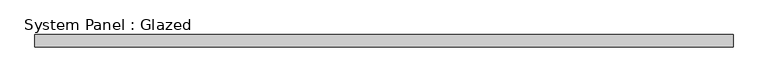
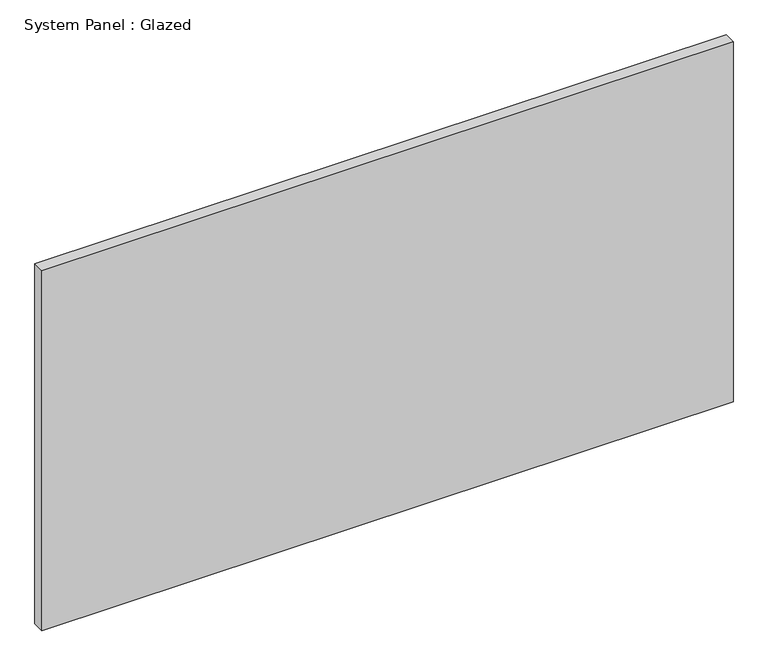
"""IFC4 building model written with IfcOpenShell, lengths in millimetres: plate geometry, System Panel : Glazed."""

from ifc_helpers import new_model, si_unit, origin, origin_with_axes, place, context, project, spatial, polyline, outline, extrude, source, transform, mapped, element, save


def system_panel_glazed_c2969f63(model_context):
    return source(origin(), model_context, "Body", "SweptSolid", [
        extrude(outline(polyline([(714.9935946, 19.05), (-714.9935946, 19.05), (-714.9935946, 44.45), (714.9935946, 44.45), (714.9935946, 19.05)])), origin_with_axes(), (0.0, 0.0, 1.0), 787.4),
    ])


if __name__ == "__main__":
    model = new_model("IFC4")
    model_context = context("Model", 3, world=origin())
    ifc_project = project(units=[si_unit("LENGTHUNIT", "METRE", prefix="MILLI")], contexts=[model_context])
    site = spatial("IfcSite", under=ifc_project)
    building = spatial("IfcBuilding", under=site)
    placement = place(None, origin())
    system_panel_glazed_shape = system_panel_glazed_c2969f63(model_context)
    element("IfcPlate", 1, ObjectType="System Panel : Glazed", at=placement, inside=building, context=model_context, shape_type="MappedRepresentation", body=[
        mapped(system_panel_glazed_shape, transform((0.0, 0.0, 0.0), x_axis=(1.0, 0.0, 0.0), y_axis=(0.0, 1.0, 0.0), z_axis=(0.0, 0.0, 1.0))),
    ])
    save(model, "model.ifc")

# Revit data of these elements
# Type "System Panel : Glazed"
#   Construction Type Id = "GSP4R"
#   Analytic Construction = "1/8 in Pilkington single glazing"
#   Visual Light Transmittance = 0.9
#   Solar Heat Gain Coefficient = 0.86
#   Heat Transfer Coefficient (U) = 1.18115 BTU/(h·ft²·°F)
#   Define Thermal Properties by = 1
# Element 1 (IfcPlate, "System Panel : Glazed")
#   Materials on its faces: "Glass"
# Materials
#   "Glass": class "Glass", colour RGB 0 128 192, transparency 0.75, Description = "Soda Lime Glass", Cost = 0
